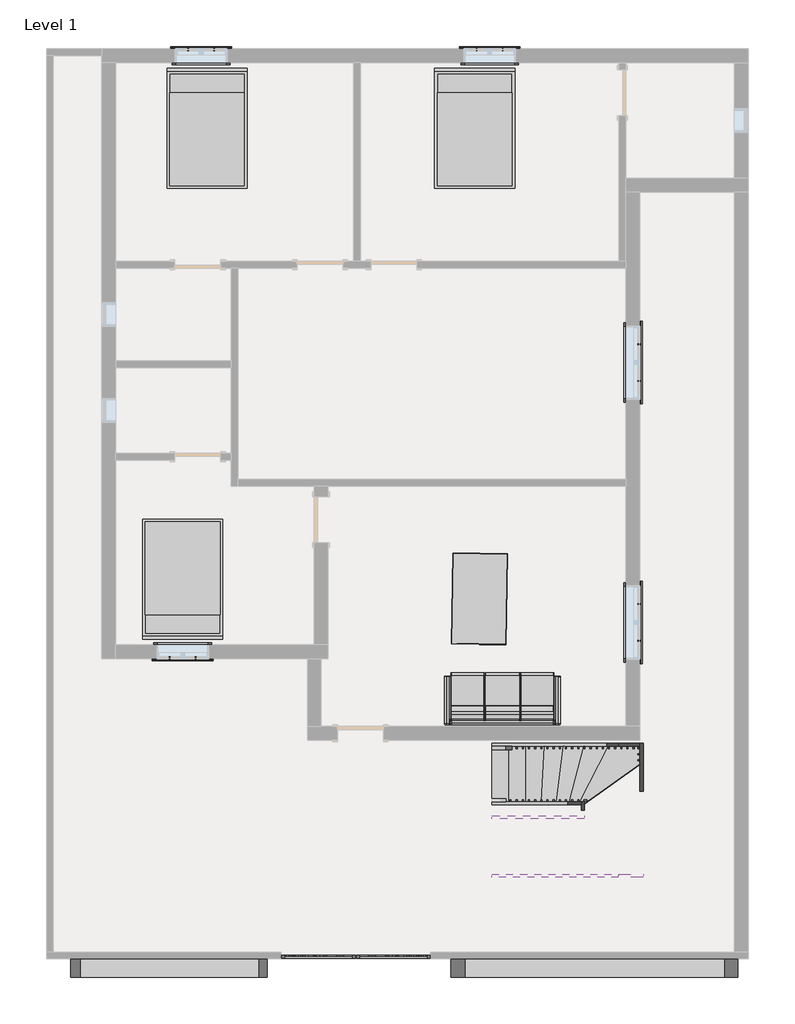
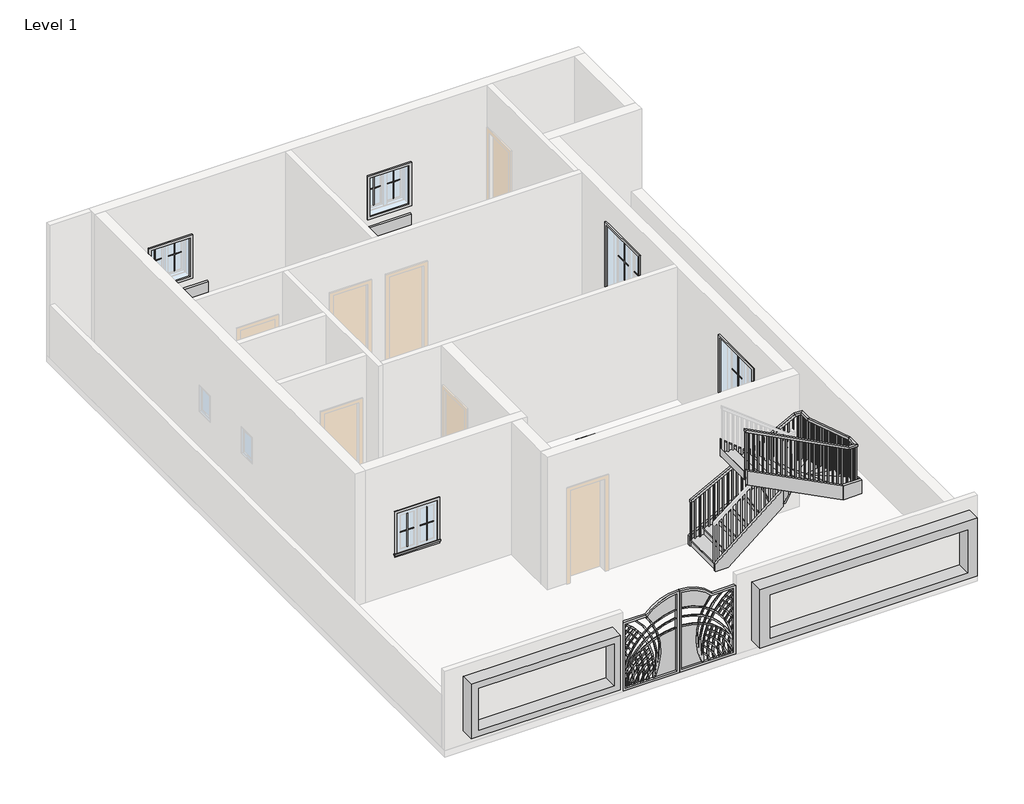
# One storey, part 2 of 2: 23 proxies, 8 members, 5 furniture elements, 1 railing, 1 stair flight.
"""IFC4 building model written with IfcOpenShell, lengths in millimetres."""

from ifc_helpers import new_model, si_unit, frame, origin, place, context, project, spatial, polyline, outline, extrude, faceted_brep, transform, mapped, element, save
from components import generic_models_6bc30956, generic_models_1_generic_models_1_5f3879a5, generic_models_2_generic_models_2_98d93cec, muntin_pattern_2x2_muntin_pattern_2x2_b3fe6957, muntin_pattern_2x2_muntin_pattern_2x2_3e0ecaf2, muntin_pattern_2x2_muntin_pattern_2x2_6dad3731, muntin_pattern_2x2_muntin_pattern_2x2_a30a3345, trim_window_exterior_flat_with_sill_41619996, trim_window_exterior_flat_with_sill_92b9b949, trim_window_interior_flat_picture_frame_51c85655, trim_window_interior_flat_picture_frame_3bb882cf, furniture_2fc85b74, furniture_29a9adb8, furniture_57072a26, bed_17739_bed_17739_15c61121, dining_table_14755_dining_table_14755_d89cb775, stair_flight_f23435a1

model = new_model("IFC4")

# Units and contexts
model_context = context("Model", 3, world=origin())
ifc_project = project(units=[si_unit("LENGTHUNIT", "METRE", prefix="MILLI")], contexts=[model_context])

# Site, building, storey
site = spatial("IfcSite", under=ifc_project)
building = spatial("IfcBuilding", under=site)
storey = spatial("IfcBuildingStorey", under=building, Name="Level 1", Elevation=0.0)

# Proxies
placement = place(None, origin())
generic_models_shape = generic_models_6bc30956(model_context)
element("IfcBuildingElementProxy", 1, Name="Generic Models", at=placement, inside=storey, context=model_context, shape_type="MappedRepresentation", body=[
    mapped(generic_models_shape, transform((-1944.195824, -6904.0064015, 0.0), x_axis=(1.0, 0.0, 0.0), y_axis=(0.0, 1.0, 0.0), z_axis=(0.0, 0.0, 1.0))),
])
generic_models_1_generic_models_1_shape = generic_models_1_generic_models_1_5f3879a5(model_context)
element("IfcBuildingElementProxy", 2, Name="Generic Models 1 : Generic Models 1", ObjectType="Generic Models 1 : Generic Models 1", at=placement, inside=storey, context=model_context, shape_type="MappedRepresentation", body=[
    mapped(generic_models_1_generic_models_1_shape, transform((0.0, 0.0, 0.0), x_axis=(1.0, 0.0, 0.0), y_axis=(0.0, 1.0, 0.0), z_axis=(0.0, 0.0, 1.0))),
])
generic_models_2_generic_models_2_shape = generic_models_2_generic_models_2_98d93cec(model_context)
element("IfcBuildingElementProxy", 3, Name="Generic Models 2 : Generic Models 2", ObjectType="Generic Models 2 : Generic Models 2", at=placement, inside=storey, context=model_context, shape_type="MappedRepresentation", body=[
    mapped(generic_models_2_generic_models_2_shape, transform((0.0, 0.0, 0.0), x_axis=(1.0, 0.0, 0.0), y_axis=(0.0, 1.0, 0.0), z_axis=(0.0, 0.0, 1.0))),
])
muntin_pattern_2x2_muntin_pattern_2x2_shape = muntin_pattern_2x2_muntin_pattern_2x2_b3fe6957(model_context)
element("IfcBuildingElementProxy", 4, Name="Muntin Pattern_2x2 : Muntin Pattern_2x2", ObjectType="Muntin Pattern_2x2 : Muntin Pattern_2x2", at=placement, inside=storey, context=model_context, shape_type="MappedRepresentation", body=[
    mapped(muntin_pattern_2x2_muntin_pattern_2x2_shape, transform((-4708.0540084, 8034.3685985, 984.25), x_axis=(1.0, 0.0, 0.0), y_axis=(0.0, 1.0, 0.0), z_axis=(0.0, 0.0, 1.0))),
])
element("IfcBuildingElementProxy", 5, Name="Muntin Pattern_2x2 : Muntin Pattern_2x2", ObjectType="Muntin Pattern_2x2 : Muntin Pattern_2x2", at=placement, inside=storey, context=model_context, shape_type="MappedRepresentation", body=[
    mapped(muntin_pattern_2x2_muntin_pattern_2x2_shape, transform((54.4459916, 8034.3685985, 984.25), x_axis=(1.0, 0.0, 0.0), y_axis=(0.0, 1.0, 0.0), z_axis=(0.0, 0.0, 1.0))),
])
element("IfcBuildingElementProxy", 6, Name="Muntin Pattern_2x2 : Muntin Pattern_2x2", ObjectType="Muntin Pattern_2x2 : Muntin Pattern_2x2", at=placement, inside=storey, context=model_context, shape_type="MappedRepresentation", body=[
    mapped(muntin_pattern_2x2_muntin_pattern_2x2_shape, transform((-4584.2290084, -2004.9814015, 984.25), x_axis=(-1.0, 0.0, 0.0), y_axis=(0.0, -1.0, 0.0), z_axis=(0.0, 0.0, 1.0))),
])
muntin_pattern_2x2_muntin_pattern_2x2_2_shape = muntin_pattern_2x2_muntin_pattern_2x2_3e0ecaf2(model_context)
element("IfcBuildingElementProxy", 7, Name="Muntin Pattern_2x2 : Muntin Pattern_2x2", ObjectType="Muntin Pattern_2x2 : Muntin Pattern_2x2", at=placement, inside=storey, context=model_context, shape_type="MappedRepresentation", body=[
    mapped(muntin_pattern_2x2_muntin_pattern_2x2_2_shape, transform((-4279.4290084, 8034.3685985, 984.25), x_axis=(-1.0, 0.0, 0.0), y_axis=(0.0, -1.0, 0.0), z_axis=(0.0, 0.0, 1.0))),
])
element("IfcBuildingElementProxy", 8, Name="Muntin Pattern_2x2 : Muntin Pattern_2x2", ObjectType="Muntin Pattern_2x2 : Muntin Pattern_2x2", at=placement, inside=storey, context=model_context, shape_type="MappedRepresentation", body=[
    mapped(muntin_pattern_2x2_muntin_pattern_2x2_2_shape, transform((483.0709916, 8034.3685985, 984.25), x_axis=(-1.0, 0.0, 0.0), y_axis=(0.0, -1.0, 0.0), z_axis=(0.0, 0.0, 1.0))),
])
element("IfcBuildingElementProxy", 9, Name="Muntin Pattern_2x2 : Muntin Pattern_2x2", ObjectType="Muntin Pattern_2x2 : Muntin Pattern_2x2", at=placement, inside=storey, context=model_context, shape_type="MappedRepresentation", body=[
    mapped(muntin_pattern_2x2_muntin_pattern_2x2_2_shape, transform((-5012.8540084, -2004.9814015, 984.25), x_axis=(1.0, 0.0, 0.0), y_axis=(0.0, 1.0, 0.0), z_axis=(0.0, 0.0, 1.0))),
])
muntin_pattern_2x2_muntin_pattern_2x2_3_shape = muntin_pattern_2x2_muntin_pattern_2x2_6dad3731(model_context)
element("IfcBuildingElementProxy", 10, Name="Muntin Pattern_2x2 : Muntin Pattern_2x2", ObjectType="Muntin Pattern_2x2 : Muntin Pattern_2x2", at=placement, inside=storey, context=model_context, shape_type="MappedRepresentation", body=[
    mapped(muntin_pattern_2x2_muntin_pattern_2x2_3_shape, transform((2735.7334916, -1114.3939015, 984.25), x_axis=(0.0, -1.0, 0.0), y_axis=(1.0, 0.0, 0.0), z_axis=(0.0, 0.0, 1.0))),
])
element("IfcBuildingElementProxy", 11, Name="Muntin Pattern_2x2 : Muntin Pattern_2x2", ObjectType="Muntin Pattern_2x2 : Muntin Pattern_2x2", at=placement, inside=storey, context=model_context, shape_type="MappedRepresentation", body=[
    mapped(muntin_pattern_2x2_muntin_pattern_2x2_3_shape, transform((2735.7334916, 3171.8560985, 984.25), x_axis=(0.0, -1.0, 0.0), y_axis=(1.0, 0.0, 0.0), z_axis=(0.0, 0.0, 1.0))),
])
muntin_pattern_2x2_muntin_pattern_2x2_4_shape = muntin_pattern_2x2_muntin_pattern_2x2_a30a3345(model_context)
element("IfcBuildingElementProxy", 12, Name="Muntin Pattern_2x2 : Muntin Pattern_2x2", ObjectType="Muntin Pattern_2x2 : Muntin Pattern_2x2", at=placement, inside=storey, context=model_context, shape_type="MappedRepresentation", body=[
    mapped(muntin_pattern_2x2_muntin_pattern_2x2_4_shape, transform((2735.7334916, -1720.8189015, 984.25), x_axis=(0.0, 1.0, 0.0), y_axis=(-1.0, 0.0, 0.0), z_axis=(0.0, 0.0, 1.0))),
])
element("IfcBuildingElementProxy", 13, Name="Muntin Pattern_2x2 : Muntin Pattern_2x2", ObjectType="Muntin Pattern_2x2 : Muntin Pattern_2x2", at=placement, inside=storey, context=model_context, shape_type="MappedRepresentation", body=[
    mapped(muntin_pattern_2x2_muntin_pattern_2x2_4_shape, transform((2735.7334916, 2565.4310985, 984.25), x_axis=(0.0, 1.0, 0.0), y_axis=(-1.0, 0.0, 0.0), z_axis=(0.0, 0.0, 1.0))),
])
trim_window_exterior_flat_with_sill_shape = trim_window_exterior_flat_with_sill_41619996(model_context)
element("IfcBuildingElementProxy", 14, Name="Trim-Window-Exterior-Flat : with Sill", ObjectType="Trim-Window-Exterior-Flat : with Sill", at=placement, inside=storey, context=model_context, shape_type="MappedRepresentation", body=[
    mapped(trim_window_exterior_flat_with_sill_shape, transform((-4493.7415084, 8043.8935985, 1828.8), x_axis=(-1.0, 0.0, 0.0), y_axis=(0.0, 0.0, 1.0), z_axis=(0.0, 1.0, 0.0))),
])
element("IfcBuildingElementProxy", 15, Name="Trim-Window-Exterior-Flat : with Sill", ObjectType="Trim-Window-Exterior-Flat : with Sill", at=placement, inside=storey, context=model_context, shape_type="MappedRepresentation", body=[
    mapped(trim_window_exterior_flat_with_sill_shape, transform((268.7584916, 8043.8935985, 1828.8), x_axis=(-1.0, 0.0, 0.0), y_axis=(0.0, 0.0, 1.0), z_axis=(0.0, 1.0, 0.0))),
])
element("IfcBuildingElementProxy", 16, Name="Trim-Window-Exterior-Flat : with Sill", ObjectType="Trim-Window-Exterior-Flat : with Sill", at=placement, inside=storey, context=model_context, shape_type="MappedRepresentation", body=[
    mapped(trim_window_exterior_flat_with_sill_shape, transform((-4798.5415084, -2014.5064015, 1828.8), x_axis=(1.0, 0.0, 0.0), y_axis=(0.0, 0.0, 1.0), z_axis=(0.0, -1.0, 0.0))),
])
trim_window_exterior_flat_with_sill_2_shape = trim_window_exterior_flat_with_sill_92b9b949(model_context)
element("IfcBuildingElementProxy", 17, Name="Trim-Window-Exterior-Flat : with Sill", ObjectType="Trim-Window-Exterior-Flat : with Sill", at=placement, inside=storey, context=model_context, shape_type="MappedRepresentation", body=[
    mapped(trim_window_exterior_flat_with_sill_2_shape, transform((2745.2584916, -1417.6064015, 2438.4), x_axis=(0.0, 1.0, 0.0), y_axis=(0.0, 0.0, 1.0), z_axis=(1.0, 0.0, 0.0))),
])
element("IfcBuildingElementProxy", 18, Name="Trim-Window-Exterior-Flat : with Sill", ObjectType="Trim-Window-Exterior-Flat : with Sill", at=placement, inside=storey, context=model_context, shape_type="MappedRepresentation", body=[
    mapped(trim_window_exterior_flat_with_sill_2_shape, transform((2745.2584916, 2868.6435985, 2438.4), x_axis=(0.0, 1.0, 0.0), y_axis=(0.0, 0.0, 1.0), z_axis=(1.0, 0.0, 0.0))),
])
trim_window_interior_flat_picture_frame_shape = trim_window_interior_flat_picture_frame_51c85655(model_context)
element("IfcBuildingElementProxy", 19, Name="Trim-Window-Interior-Flat : Picture Frame", ObjectType="Trim-Window-Interior-Flat : Picture Frame", at=placement, inside=storey, context=model_context, shape_type="MappedRepresentation", body=[
    mapped(trim_window_interior_flat_picture_frame_shape, transform((-4493.7415084, 7815.2935985, 1828.8), x_axis=(1.0, 0.0, 0.0), y_axis=(0.0, 0.0, 1.0), z_axis=(0.0, -1.0, 0.0))),
])
element("IfcBuildingElementProxy", 20, Name="Trim-Window-Interior-Flat : Picture Frame", ObjectType="Trim-Window-Interior-Flat : Picture Frame", at=placement, inside=storey, context=model_context, shape_type="MappedRepresentation", body=[
    mapped(trim_window_interior_flat_picture_frame_shape, transform((268.7584916, 7815.2935985, 1828.8), x_axis=(1.0, 0.0, 0.0), y_axis=(0.0, 0.0, 1.0), z_axis=(0.0, -1.0, 0.0))),
])
element("IfcBuildingElementProxy", 21, Name="Trim-Window-Interior-Flat : Picture Frame", ObjectType="Trim-Window-Interior-Flat : Picture Frame", at=placement, inside=storey, context=model_context, shape_type="MappedRepresentation", body=[
    mapped(trim_window_interior_flat_picture_frame_shape, transform((-4798.5415084, -1785.9064015, 1828.8), x_axis=(-1.0, 0.0, 0.0), y_axis=(0.0, 0.0, 1.0), z_axis=(0.0, 1.0, 0.0))),
])
trim_window_interior_flat_picture_frame_2_shape = trim_window_interior_flat_picture_frame_3bb882cf(model_context)
element("IfcBuildingElementProxy", 22, Name="Trim-Window-Interior-Flat : Picture Frame", ObjectType="Trim-Window-Interior-Flat : Picture Frame", at=placement, inside=storey, context=model_context, shape_type="MappedRepresentation", body=[
    mapped(trim_window_interior_flat_picture_frame_2_shape, transform((2516.6584916, -1417.6064015, 2438.4), x_axis=(0.0, -1.0, 0.0), y_axis=(0.0, 0.0, 1.0), z_axis=(-1.0, 0.0, 0.0))),
])
element("IfcBuildingElementProxy", 23, Name="Trim-Window-Interior-Flat : Picture Frame", ObjectType="Trim-Window-Interior-Flat : Picture Frame", at=placement, inside=storey, context=model_context, shape_type="MappedRepresentation", body=[
    mapped(trim_window_interior_flat_picture_frame_2_shape, transform((2516.6584916, 2868.6435985, 2438.4), x_axis=(0.0, -1.0, 0.0), y_axis=(0.0, 0.0, 1.0), z_axis=(-1.0, 0.0, 0.0))),
])

# Furniture
furniture_shape = furniture_2fc85b74(model_context)
furniture_2_shape = furniture_29a9adb8(model_context)
furniture_3_shape = furniture_57072a26(model_context)
element("IfcFurniture", 24, at=placement, inside=storey, context=model_context, shape_type="MappedRepresentation", body=[
    mapped(furniture_shape, transform((477.9947981, -2301.7922014, 0.0), x_axis=(-1.0, 0.0, 0.0), y_axis=(0.0, -1.0, 0.0), z_axis=(0.0, 0.0, 1.0))),
    mapped(furniture_2_shape, transform((477.9947981, -2301.7922014, 0.0), x_axis=(-1.0, 0.0, 0.0), y_axis=(0.0, -1.0, 0.0), z_axis=(0.0, 0.0, 1.0))),
    mapped(furniture_3_shape, transform((477.9947981, -2301.7922014, 0.0), x_axis=(-1.0, 0.0, 0.0), y_axis=(0.0, -1.0, 0.0), z_axis=(0.0, 0.0, 1.0))),
])
bed_17739_bed_17739_shape = bed_17739_bed_17739_15c61121(model_context)
element("IfcFurniture", 25, ObjectType="Bed_17739 : Bed_17739", at=placement, inside=storey, context=model_context, shape_type="MappedRepresentation", body=[
    mapped(bed_17739_bed_17739_shape, transform((-4398.4915084, 6710.3935985, 0.0), x_axis=(1.0, 0.0, 0.0), y_axis=(0.0, 1.0, 0.0), z_axis=(0.0, 0.0, 1.0))),
])
element("IfcFurniture", 26, ObjectType="Bed_17739 : Bed_17739", at=placement, inside=storey, context=model_context, shape_type="MappedRepresentation", body=[
    mapped(bed_17739_bed_17739_shape, transform((21.1084916, 6710.3935985, 0.0), x_axis=(1.0, 0.0, 0.0), y_axis=(0.0, 1.0, 0.0), z_axis=(0.0, 0.0, 1.0))),
])
element("IfcFurniture", 27, ObjectType="Bed_17739 : Bed_17739", at=placement, inside=storey, context=model_context, shape_type="MappedRepresentation", body=[
    mapped(bed_17739_bed_17739_shape, transform((-4798.5415084, -681.0064015, 0.0), x_axis=(-1.0, 0.0, 0.0), y_axis=(0.0, -1.0, 0.0), z_axis=(0.0, 0.0, 1.0))),
])
dining_table_14755_dining_table_14755_shape = dining_table_14755_dining_table_14755_d89cb775(model_context)
element("IfcFurniture", 28, ObjectType="Dining_table_14755 : Dining_table_14755", at=placement, inside=storey, context=model_context, shape_type="MappedRepresentation", body=[
    mapped(dining_table_14755_dining_table_14755_shape, transform((535.647979, -1785.9064015, 0.0), x_axis=(0.016088397262737867, 0.9998705733611308, 0.0), y_axis=(-0.9998705733611308, 0.016088397262737867, 0.0), z_axis=(0.0, 0.0, 1.0))),
])

# Members
element("IfcMember", 29, ObjectType="Stringer - 2\" Width", at=placement, inside=storey, context=model_context, shape_type="SweptSolid", body=[
    extrude(outline(polyline([(229.639954, 306.9570026), (0.0, 306.9570026), (0.0, 526.7193201), (962.500629, 2394.3741942), (1305.3956453, 2394.3741942), (229.639954, 306.9570026)])), frame((0.0, -3462.3064015, 0.0), z_axis=(0.0, 1.0, 0.0), x_axis=(0.0, 0.0, 1.0)), (0.0, 0.0, 1.0), 50.8),
])
element("IfcMember", 30, ObjectType="Stringer - 2\" Width", at=placement, inside=storey, context=model_context, shape_type="SweptSolid", body=[
    extrude(outline(polyline([(2394.3741942, -3462.3064015), (2394.3741942, -3411.5064015), (2749.0886944, -3411.5064015), (2749.0886944, -3462.3064015), (2394.3741942, -3462.3064015)])), frame((0.0, 0.0, 962.500629), z_axis=(0.0, 0.0, 1.0), x_axis=(1.0, 0.0, 0.0)), (0.0, 0.0, 1.0), 342.8950162),
])
element("IfcMember", 31, ObjectType="Stringer - 2\" Width", at=placement, inside=storey, context=model_context, shape_type="SweptSolid", body=[
    extrude(outline(polyline([(-3411.5064015, 1289.0952212), (-3411.5064015, 1000.5956453), (-3581.0288845, 1000.5956453), (-5570.5064015, 1638.9682298), (-5570.5064015, 1969.9972697), (-5533.5262842, 1969.9972697), (-3411.5064015, 1289.0952212)])), frame((2749.0886944, 0.0, 0.0), z_axis=(1.0, 0.0, 0.0), x_axis=(0.0, 1.0, 0.0)), (0.0, 0.0, 1.0), 50.8),
])
element("IfcMember", 32, ObjectType="Stringer - 2\" Width", at=placement, inside=storey, context=model_context, shape_type="SweptSolid", body=[
    extrude(outline(polyline([(2799.8886944, -5570.5064015), (2799.8886944, -5621.3064015), (2394.3741942, -5621.3064015), (2394.3741942, -5570.5064015), (2799.8886944, -5570.5064015)])), frame((0.0, 0.0, 1649.8904473), z_axis=(0.0, 0.0, 1.0), x_axis=(1.0, 0.0, 0.0)), (0.0, 0.0, 1.0), 320.1068224),
])
element("IfcMember", 33, ObjectType="Stringer - 2\" Width", at=placement, inside=storey, context=model_context, shape_type="SweptSolid", body=[
    extrude(outline(polyline([(1649.8904473, 2394.3741942), (1969.9972697, 2394.3741942), (3045.7529609, 306.9570026), (2725.6461385, 306.9570026), (1649.8904473, 2394.3741942)])), frame((0.0, -5621.3064015, 0.0), z_axis=(0.0, 1.0, 0.0), x_axis=(0.0, 0.0, 1.0)), (0.0, 0.0, 1.0), 50.8),
])
element("IfcMember", 34, ObjectType="Stringer - 2\" Width", at=placement, inside=storey, context=model_context, shape_type="SweptSolid", body=[
    extrude(outline(polyline([(176.1764461, 306.9570026), (0.0, 306.9570026), (0.0, 573.2186471), (987.1410923, 1783.8886944), (1380.418648, 1783.8886944), (176.1764461, 306.9570026)])), frame((0.0, -4427.5064015, 0.0), z_axis=(0.0, 1.0, 0.0), x_axis=(0.0, 0.0, 1.0)), (0.0, 0.0, 1.0), 50.8),
])
element("IfcMember", 35, ObjectType="Stringer - 2\" Width", at=placement, inside=storey, context=model_context, shape_type="SweptSolid", body=[
    extrude(outline(polyline([(-4376.7064015, 1573.2682978), (-4376.7064015, 1028.5617647), (-4410.9486188, 1028.5617647), (-4605.3064015, 1360.465107), (-4605.3064015, 1926.1409689), (-4583.3435189, 1926.1409689), (-4376.7064015, 1573.2682978)])), frame((1783.8886944, 0.0, 0.0), z_axis=(1.0, 0.0, 0.0), x_axis=(0.0, 1.0, 0.0)), (0.0, 0.0, 1.0), 50.8),
])
element("IfcMember", 36, ObjectType="Stringer - 2\" Width", at=placement, inside=storey, context=model_context, shape_type="SweptSolid", body=[
    extrude(outline(polyline([(1532.8634131, 1834.6886944), (1926.1409689, 1834.6886944), (3171.8038432, 306.9570026), (2778.5262875, 306.9570026), (1532.8634131, 1834.6886944)])), frame((0.0, -4656.1064015, 0.0), z_axis=(0.0, 1.0, 0.0), x_axis=(0.0, 0.0, 1.0)), (0.0, 0.0, 1.0), 50.8),
])

# Railing
element("IfcRailing", 37, ObjectType="Handrail - Rectangular", at=placement, inside=storey, context=model_context, shape_type="SolidModel", body=[
    faceted_brep([(306.9570026, -3462.3064015, 1083.7333333), (306.9570026, -3462.3064015, 1026.2742652), (306.9570026, -3513.1064015, 1026.2742652), (306.9570026, -3513.1064015, 1083.7333333), (2564.6820646, -3462.3064015, 2277.0239201), (2577.2811291, -3462.3064015, 2226.2239201), (2577.2811291, -3513.1064015, 2226.2239201), (2564.6820646, -3513.1064015, 2277.0239201), (2749.0886944, -3462.3064015, 2277.0239201), (2749.0886944, -3462.3064015, 2226.2239201), (2698.2886944, -3513.1064015, 2226.2239201), (2698.2886944, -3513.1064015, 2277.0239201), (2749.0886944, -3749.6182836, 2277.0239201), (2749.0886944, -3757.5688598, 2226.2239201), (2698.2886944, -3757.5688598, 2226.2239201), (2698.2886944, -3749.6182836, 2277.0239201), (2749.0886944, -5283.1945194, 2769.1094132), (2749.0886944, -5291.1450955, 2718.3094132), (2698.2886944, -5291.1450955, 2718.3094132), (2698.2886944, -5283.1945194, 2769.1094132), (2749.0886944, -5570.5064015, 2769.1094132), (2749.0886944, -5570.5064015, 2718.3094132), (2698.2886944, -5519.7064015, 2718.3094132), (2698.2886944, -5519.7064015, 2769.1094132), (2564.6820646, -5570.5064015, 2769.1094132), (2552.0830001, -5570.5064015, 2718.3094132), (2552.0830001, -5519.7064015, 2718.3094132), (2564.6820646, -5519.7064015, 2769.1094132), (306.9570026, -5570.5064015, 3962.4), (306.9570026, -5519.7064015, 3962.4), (306.9570026, -5519.7064015, 3904.9409318), (306.9570026, -5570.5064015, 3904.9409318)], [[[0, 1, 2, 3]], [[1, 0, 4, 5]], [[2, 1, 5, 6]], [[3, 2, 6, 7]], [[0, 3, 7, 4]], [[5, 4, 8, 9]], [[6, 5, 9, 10]], [[7, 6, 10, 11]], [[4, 7, 11, 8]], [[9, 8, 12, 13]], [[10, 9, 13, 14]], [[11, 10, 14, 15]], [[8, 11, 15, 12]], [[13, 12, 16, 17]], [[14, 13, 17, 18]], [[15, 14, 18, 19]], [[12, 15, 19, 16]], [[17, 16, 20, 21]], [[18, 17, 21, 22]], [[19, 18, 22, 23]], [[16, 19, 23, 20]], [[21, 20, 24, 25]], [[22, 21, 25, 26]], [[23, 22, 26, 27]], [[20, 23, 27, 24]], [[28, 29, 30, 31]], [[25, 24, 28, 31]], [[26, 25, 31, 30]], [[27, 26, 30, 29]], [[24, 27, 29, 28]]]),
    extrude(outline(polyline([(3867.7284102, 377.3636944), (2878.6666667, 377.3636944), (2878.6666667, 396.4136944), (3857.6597858, 396.4136944), (3867.7284102, 377.3636944)])), frame((0.0, -5554.6314015, 0.0), z_axis=(0.0, 1.0, 0.0), x_axis=(0.0, 0.0, 1.0)), (0.0, 0.0, 1.0), 19.05),
    extrude(outline(polyline([(3814.02908, 478.9636944), (2878.6666667, 478.9636944), (2878.6666667, 498.0136944), (3803.9604556, 498.0136944), (3814.02908, 478.9636944)])), frame((0.0, -5554.6314015, 0.0), z_axis=(0.0, 1.0, 0.0), x_axis=(0.0, 0.0, 1.0)), (0.0, 0.0, 1.0), 19.05),
    extrude(outline(polyline([(3760.3297498, 580.5636944), (2709.3333333, 580.5636944), (2709.3333333, 599.6136944), (3750.2611254, 599.6136944), (3760.3297498, 580.5636944)])), frame((0.0, -5554.6314015, 0.0), z_axis=(0.0, 1.0, 0.0), x_axis=(0.0, 0.0, 1.0)), (0.0, 0.0, 1.0), 19.05),
    extrude(outline(polyline([(3706.6304196, 682.1636944), (2709.3333333, 682.1636944), (2709.3333333, 701.2136944), (3696.5617952, 701.2136944), (3706.6304196, 682.1636944)])), frame((0.0, -5554.6314015, 0.0), z_axis=(0.0, 1.0, 0.0), x_axis=(0.0, 0.0, 1.0)), (0.0, 0.0, 1.0), 19.05),
    extrude(outline(polyline([(3652.9310894, 783.7636944), (2709.3333333, 783.7636944), (2709.3333333, 802.8136944), (3642.862465, 802.8136944), (3652.9310894, 783.7636944)])), frame((0.0, -5554.6314015, 0.0), z_axis=(0.0, 1.0, 0.0), x_axis=(0.0, 0.0, 1.0)), (0.0, 0.0, 1.0), 19.05),
    extrude(outline(polyline([(3599.2317592, 885.3636944), (2540.0, 885.3636944), (2540.0, 904.4136944), (3589.1631348, 904.4136944), (3599.2317592, 885.3636944)])), frame((0.0, -5554.6314015, 0.0), z_axis=(0.0, 1.0, 0.0), x_axis=(0.0, 0.0, 1.0)), (0.0, 0.0, 1.0), 19.05),
    extrude(outline(polyline([(3545.532429, 986.9636944), (2540.0, 986.9636944), (2540.0, 1006.0136944), (3535.4638046, 1006.0136944), (3545.532429, 986.9636944)])), frame((0.0, -5554.6314015, 0.0), z_axis=(0.0, 1.0, 0.0), x_axis=(0.0, 0.0, 1.0)), (0.0, 0.0, 1.0), 19.05),
    extrude(outline(polyline([(3491.8330988, 1088.5636944), (2540.0, 1088.5636944), (2540.0, 1107.6136944), (3481.7644744, 1107.6136944), (3491.8330988, 1088.5636944)])), frame((0.0, -5554.6314015, 0.0), z_axis=(0.0, 1.0, 0.0), x_axis=(0.0, 0.0, 1.0)), (0.0, 0.0, 1.0), 19.05),
    extrude(outline(polyline([(3438.1337686, 1190.1636944), (2370.6666667, 1190.1636944), (2370.6666667, 1209.2136944), (3428.0651442, 1209.2136944), (3438.1337686, 1190.1636944)])), frame((0.0, -5554.6314015, 0.0), z_axis=(0.0, 1.0, 0.0), x_axis=(0.0, 0.0, 1.0)), (0.0, 0.0, 1.0), 19.05),
    extrude(outline(polyline([(3384.4344384, 1291.7636944), (2370.6666667, 1291.7636944), (2370.6666667, 1310.8136944), (3374.365814, 1310.8136944), (3384.4344384, 1291.7636944)])), frame((0.0, -5554.6314015, 0.0), z_axis=(0.0, 1.0, 0.0), x_axis=(0.0, 0.0, 1.0)), (0.0, 0.0, 1.0), 19.05),
    extrude(outline(polyline([(3330.7351082, 1393.3636944), (2370.6666667, 1393.3636944), (2370.6666667, 1412.4136944), (3320.6664838, 1412.4136944), (3330.7351082, 1393.3636944)])), frame((0.0, -5554.6314015, 0.0), z_axis=(0.0, 1.0, 0.0), x_axis=(0.0, 0.0, 1.0)), (0.0, 0.0, 1.0), 19.05),
    extrude(outline(polyline([(3277.035778, 1494.9636944), (2201.3333333, 1494.9636944), (2201.3333333, 1514.0136944), (3266.9671536, 1514.0136944), (3277.035778, 1494.9636944)])), frame((0.0, -5554.6314015, 0.0), z_axis=(0.0, 1.0, 0.0), x_axis=(0.0, 0.0, 1.0)), (0.0, 0.0, 1.0), 19.05),
    extrude(outline(polyline([(3223.3364478, 1596.5636944), (2201.3333333, 1596.5636944), (2201.3333333, 1615.6136944), (3213.2678234, 1615.6136944), (3223.3364478, 1596.5636944)])), frame((0.0, -5554.6314015, 0.0), z_axis=(0.0, 1.0, 0.0), x_axis=(0.0, 0.0, 1.0)), (0.0, 0.0, 1.0), 19.05),
    extrude(outline(polyline([(3169.6371176, 1698.1636944), (2201.3333333, 1698.1636944), (2201.3333333, 1717.2136944), (3159.5684932, 1717.2136944), (3169.6371176, 1698.1636944)])), frame((0.0, -5554.6314015, 0.0), z_axis=(0.0, 1.0, 0.0), x_axis=(0.0, 0.0, 1.0)), (0.0, 0.0, 1.0), 19.05),
    extrude(outline(polyline([(3115.9377874, 1799.7636944), (2201.3333333, 1799.7636944), (2201.3333333, 1818.8136944), (3105.869163, 1818.8136944), (3115.9377874, 1799.7636944)])), frame((0.0, -5554.6314015, 0.0), z_axis=(0.0, 1.0, 0.0), x_axis=(0.0, 0.0, 1.0)), (0.0, 0.0, 1.0), 19.05),
    extrude(outline(polyline([(3062.2384572, 1901.3636944), (2032.0, 1901.3636944), (2032.0, 1920.4136944), (3052.1698328, 1920.4136944), (3062.2384572, 1901.3636944)])), frame((0.0, -5554.6314015, 0.0), z_axis=(0.0, 1.0, 0.0), x_axis=(0.0, 0.0, 1.0)), (0.0, 0.0, 1.0), 19.05),
    extrude(outline(polyline([(3008.539127, 2002.9636944), (2032.0, 2002.9636944), (2032.0, 2022.0136944), (2998.4705026, 2022.0136944), (3008.539127, 2002.9636944)])), frame((0.0, -5554.6314015, 0.0), z_axis=(0.0, 1.0, 0.0), x_axis=(0.0, 0.0, 1.0)), (0.0, 0.0, 1.0), 19.05),
    extrude(outline(polyline([(2954.8397968, 2104.5636944), (2032.0, 2104.5636944), (2032.0, 2123.6136944), (2944.7711724, 2123.6136944), (2954.8397968, 2104.5636944)])), frame((0.0, -5554.6314015, 0.0), z_axis=(0.0, 1.0, 0.0), x_axis=(0.0, 0.0, 1.0)), (0.0, 0.0, 1.0), 19.05),
    extrude(outline(polyline([(2901.1404666, 2206.1636944), (2032.0, 2206.1636944), (2032.0, 2225.2136944), (2891.0718422, 2225.2136944), (2901.1404666, 2206.1636944)])), frame((0.0, -5554.6314015, 0.0), z_axis=(0.0, 1.0, 0.0), x_axis=(0.0, 0.0, 1.0)), (0.0, 0.0, 1.0), 19.05),
    extrude(outline(polyline([(2847.4411364, 2307.7636944), (1862.6666667, 2307.7636944), (1862.6666667, 2326.8136944), (2837.372512, 2326.8136944), (2847.4411364, 2307.7636944)])), frame((0.0, -5554.6314015, 0.0), z_axis=(0.0, 1.0, 0.0), x_axis=(0.0, 0.0, 1.0)), (0.0, 0.0, 1.0), 19.05),
    extrude(outline(polyline([(2793.7418062, 2409.3636944), (1862.6666667, 2409.3636944), (1862.6666667, 2428.4136944), (2783.6731818, 2428.4136944), (2793.7418062, 2409.3636944)])), frame((0.0, -5554.6314015, 0.0), z_axis=(0.0, 1.0, 0.0), x_axis=(0.0, 0.0, 1.0)), (0.0, 0.0, 1.0), 19.05),
    extrude(outline(polyline([(2740.042476, 2510.9636944), (1862.6666667, 2510.9636944), (1862.6666667, 2530.0136944), (2729.9738516, 2530.0136944), (2740.042476, 2510.9636944)])), frame((0.0, -5554.6314015, 0.0), z_axis=(0.0, 1.0, 0.0), x_axis=(0.0, 0.0, 1.0)), (0.0, 0.0, 1.0), 19.05),
    extrude(outline(polyline([(2631.6136944, -5554.6314015), (2612.5636944, -5554.6314015), (2612.5636944, -5535.5814015), (2631.6136944, -5535.5814015), (2631.6136944, -5554.6314015)])), frame((0.0, 0.0, 1862.6666667), z_axis=(0.0, 0.0, 1.0), x_axis=(1.0, 0.0, 0.0)), (0.0, 0.0, 1.0), 855.6427466),
    extrude(outline(polyline([(2733.2136944, -5510.1814015), (2733.2136944, -5529.2314015), (2714.1636944, -5529.2314015), (2714.1636944, -5510.1814015), (2733.2136944, -5510.1814015)])), frame((0.0, 0.0, 1862.6666667), z_axis=(0.0, 0.0, 1.0), x_axis=(1.0, 0.0, 0.0)), (0.0, 0.0, 1.0), 855.6427466),
    extrude(outline(polyline([(2733.2136944, -5408.5814015), (2733.2136944, -5427.6314015), (2714.1636944, -5427.6314015), (2714.1636944, -5408.5814015), (2733.2136944, -5408.5814015)])), frame((0.0, 0.0, 1862.6666667), z_axis=(0.0, 0.0, 1.0), x_axis=(1.0, 0.0, 0.0)), (0.0, 0.0, 1.0), 855.6427466),
    extrude(outline(polyline([(2733.2136944, -5306.9814015), (2733.2136944, -5326.0314015), (2714.1636944, -5326.0314015), (2714.1636944, -5306.9814015), (2733.2136944, -5306.9814015)])), frame((0.0, 0.0, 1862.6666667), z_axis=(0.0, 0.0, 1.0), x_axis=(1.0, 0.0, 0.0)), (0.0, 0.0, 1.0), 855.6427466),
    extrude(outline(polyline([(-5205.3814015, 2690.7900316), (-5205.3814015, 1693.3333333), (-5224.4314015, 1693.3333333), (-5224.4314015, 2696.9026907), (-5205.3814015, 2690.7900316)])), frame((2714.1636944, 0.0, 0.0), z_axis=(1.0, 0.0, 0.0), x_axis=(0.0, 1.0, 0.0)), (0.0, 0.0, 1.0), 19.05),
    extrude(outline(polyline([(-5103.7814015, 2658.1891834), (-5103.7814015, 1693.3333333), (-5122.8314015, 1693.3333333), (-5122.8314015, 2664.3018425), (-5103.7814015, 2658.1891834)])), frame((2714.1636944, 0.0, 0.0), z_axis=(1.0, 0.0, 0.0), x_axis=(0.0, 1.0, 0.0)), (0.0, 0.0, 1.0), 19.05),
    extrude(outline(polyline([(-5002.1814015, 2625.5883352), (-5002.1814015, 1693.3333333), (-5021.2314015, 1693.3333333), (-5021.2314015, 2631.7009942), (-5002.1814015, 2625.5883352)])), frame((2714.1636944, 0.0, 0.0), z_axis=(1.0, 0.0, 0.0), x_axis=(0.0, 1.0, 0.0)), (0.0, 0.0, 1.0), 19.05),
    extrude(outline(polyline([(-4900.5814015, 2592.987487), (-4900.5814015, 1693.3333333), (-4919.6314015, 1693.3333333), (-4919.6314015, 2599.100146), (-4900.5814015, 2592.987487)])), frame((2714.1636944, 0.0, 0.0), z_axis=(1.0, 0.0, 0.0), x_axis=(0.0, 1.0, 0.0)), (0.0, 0.0, 1.0), 19.05),
    extrude(outline(polyline([(-4798.9814015, 2560.3866387), (-4798.9814015, 1693.3333333), (-4818.0314015, 1693.3333333), (-4818.0314015, 2566.4992978), (-4798.9814015, 2560.3866387)])), frame((2714.1636944, 0.0, 0.0), z_axis=(1.0, 0.0, 0.0), x_axis=(0.0, 1.0, 0.0)), (0.0, 0.0, 1.0), 19.05),
    extrude(outline(polyline([(-4697.3814015, 2527.7857905), (-4697.3814015, 1524.0), (-4716.4314015, 1524.0), (-4716.4314015, 2533.8984495), (-4697.3814015, 2527.7857905)])), frame((2714.1636944, 0.0, 0.0), z_axis=(1.0, 0.0, 0.0), x_axis=(0.0, 1.0, 0.0)), (0.0, 0.0, 1.0), 19.05),
    extrude(outline(polyline([(-4595.7814015, 2495.1849423), (-4595.7814015, 1524.0), (-4614.8314015, 1524.0), (-4614.8314015, 2501.2976013), (-4595.7814015, 2495.1849423)])), frame((2714.1636944, 0.0, 0.0), z_axis=(1.0, 0.0, 0.0), x_axis=(0.0, 1.0, 0.0)), (0.0, 0.0, 1.0), 19.05),
    extrude(outline(polyline([(-4494.1814015, 2462.5840941), (-4494.1814015, 1524.0), (-4513.2314015, 1524.0), (-4513.2314015, 2468.6967531), (-4494.1814015, 2462.5840941)])), frame((2714.1636944, 0.0, 0.0), z_axis=(1.0, 0.0, 0.0), x_axis=(0.0, 1.0, 0.0)), (0.0, 0.0, 1.0), 19.05),
    extrude(outline(polyline([(-4392.5814015, 2429.9832458), (-4392.5814015, 1524.0), (-4411.6314015, 1524.0), (-4411.6314015, 2436.0959049), (-4392.5814015, 2429.9832458)])), frame((2714.1636944, 0.0, 0.0), z_axis=(1.0, 0.0, 0.0), x_axis=(0.0, 1.0, 0.0)), (0.0, 0.0, 1.0), 19.05),
    extrude(outline(polyline([(-4290.9814015, 2397.3823976), (-4290.9814015, 1524.0), (-4310.0314015, 1524.0), (-4310.0314015, 2403.4950566), (-4290.9814015, 2397.3823976)])), frame((2714.1636944, 0.0, 0.0), z_axis=(1.0, 0.0, 0.0), x_axis=(0.0, 1.0, 0.0)), (0.0, 0.0, 1.0), 19.05),
    extrude(outline(polyline([(-4189.3814015, 2364.7815494), (-4189.3814015, 1354.6666667), (-4208.4314015, 1354.6666667), (-4208.4314015, 2370.8942084), (-4189.3814015, 2364.7815494)])), frame((2714.1636944, 0.0, 0.0), z_axis=(1.0, 0.0, 0.0), x_axis=(0.0, 1.0, 0.0)), (0.0, 0.0, 1.0), 19.05),
    extrude(outline(polyline([(-4087.7814015, 2332.1807011), (-4087.7814015, 1354.6666667), (-4106.8314015, 1354.6666667), (-4106.8314015, 2338.2933602), (-4087.7814015, 2332.1807011)])), frame((2714.1636944, 0.0, 0.0), z_axis=(1.0, 0.0, 0.0), x_axis=(0.0, 1.0, 0.0)), (0.0, 0.0, 1.0), 19.05),
    extrude(outline(polyline([(-3986.1814015, 2299.5798529), (-3986.1814015, 1354.6666667), (-4005.2314015, 1354.6666667), (-4005.2314015, 2305.692512), (-3986.1814015, 2299.5798529)])), frame((2714.1636944, 0.0, 0.0), z_axis=(1.0, 0.0, 0.0), x_axis=(0.0, 1.0, 0.0)), (0.0, 0.0, 1.0), 19.05),
    extrude(outline(polyline([(-3884.5814015, 2266.9790047), (-3884.5814015, 1354.6666667), (-3903.6314015, 1354.6666667), (-3903.6314015, 2273.0916637), (-3884.5814015, 2266.9790047)])), frame((2714.1636944, 0.0, 0.0), z_axis=(1.0, 0.0, 0.0), x_axis=(0.0, 1.0, 0.0)), (0.0, 0.0, 1.0), 19.05),
    extrude(outline(polyline([(-3782.9814015, 2234.3781565), (-3782.9814015, 1354.6666667), (-3802.0314015, 1354.6666667), (-3802.0314015, 2240.4908155), (-3782.9814015, 2234.3781565)])), frame((2714.1636944, 0.0, 0.0), z_axis=(1.0, 0.0, 0.0), x_axis=(0.0, 1.0, 0.0)), (0.0, 0.0, 1.0), 19.05),
    extrude(outline(polyline([(2733.2136944, -3681.3814015), (2733.2136944, -3700.4314015), (2714.1636944, -3700.4314015), (2714.1636944, -3681.3814015), (2733.2136944, -3681.3814015)])), frame((0.0, 0.0, 1185.3333333), z_axis=(0.0, 0.0, 1.0), x_axis=(1.0, 0.0, 0.0)), (0.0, 0.0, 1.0), 1040.8905868),
    extrude(outline(polyline([(2733.2136944, -3579.7814015), (2733.2136944, -3598.8314015), (2714.1636944, -3598.8314015), (2714.1636944, -3579.7814015), (2733.2136944, -3579.7814015)])), frame((0.0, 0.0, 1185.3333333), z_axis=(0.0, 0.0, 1.0), x_axis=(1.0, 0.0, 0.0)), (0.0, 0.0, 1.0), 1040.8905868),
    extrude(outline(polyline([(2634.2320026, -3478.1814015), (2653.2820026, -3478.1814015), (2653.2820026, -3497.2314015), (2634.2320026, -3497.2314015), (2634.2320026, -3478.1814015)])), frame((0.0, 0.0, 1185.3333333), z_axis=(0.0, 0.0, 1.0), x_axis=(1.0, 0.0, 0.0)), (0.0, 0.0, 1.0), 1040.8905868),
    extrude(outline(polyline([(2202.6252174, 2532.6320026), (1185.3333333, 2532.6320026), (1185.3333333, 2551.6820026), (2212.6938418, 2551.6820026), (2202.6252174, 2532.6320026)])), frame((0.0, -3497.2314015, 0.0), z_axis=(0.0, 1.0, 0.0), x_axis=(0.0, 0.0, 1.0)), (0.0, 0.0, 1.0), 19.05),
    extrude(outline(polyline([(2148.9258872, 2431.0320026), (1185.3333333, 2431.0320026), (1185.3333333, 2450.0820026), (2158.9945116, 2450.0820026), (2148.9258872, 2431.0320026)])), frame((0.0, -3497.2314015, 0.0), z_axis=(0.0, 1.0, 0.0), x_axis=(0.0, 0.0, 1.0)), (0.0, 0.0, 1.0), 19.05),
    extrude(outline(polyline([(2095.226557, 2329.4320026), (1185.3333333, 2329.4320026), (1185.3333333, 2348.4820026), (2105.2951814, 2348.4820026), (2095.226557, 2329.4320026)])), frame((0.0, -3497.2314015, 0.0), z_axis=(0.0, 1.0, 0.0), x_axis=(0.0, 0.0, 1.0)), (0.0, 0.0, 1.0), 19.05),
    extrude(outline(polyline([(2041.5272268, 2227.8320026), (1185.3333333, 2227.8320026), (1185.3333333, 2246.8820026), (2051.5958512, 2246.8820026), (2041.5272268, 2227.8320026)])), frame((0.0, -3497.2314015, 0.0), z_axis=(0.0, 1.0, 0.0), x_axis=(0.0, 0.0, 1.0)), (0.0, 0.0, 1.0), 19.05),
    extrude(outline(polyline([(1987.8278966, 2126.2320026), (1016.0, 2126.2320026), (1016.0, 2145.2820026), (1997.896521, 2145.2820026), (1987.8278966, 2126.2320026)])), frame((0.0, -3497.2314015, 0.0), z_axis=(0.0, 1.0, 0.0), x_axis=(0.0, 0.0, 1.0)), (0.0, 0.0, 1.0), 19.05),
    extrude(outline(polyline([(1934.1285664, 2024.6320026), (1016.0, 2024.6320026), (1016.0, 2043.6820026), (1944.1971908, 2043.6820026), (1934.1285664, 2024.6320026)])), frame((0.0, -3497.2314015, 0.0), z_axis=(0.0, 1.0, 0.0), x_axis=(0.0, 0.0, 1.0)), (0.0, 0.0, 1.0), 19.05),
    extrude(outline(polyline([(1880.4292362, 1923.0320026), (1016.0, 1923.0320026), (1016.0, 1942.0820026), (1890.4978606, 1942.0820026), (1880.4292362, 1923.0320026)])), frame((0.0, -3497.2314015, 0.0), z_axis=(0.0, 1.0, 0.0), x_axis=(0.0, 0.0, 1.0)), (0.0, 0.0, 1.0), 19.05),
    extrude(outline(polyline([(1826.729906, 1821.4320026), (1016.0, 1821.4320026), (1016.0, 1840.4820026), (1836.7985304, 1840.4820026), (1826.729906, 1821.4320026)])), frame((0.0, -3497.2314015, 0.0), z_axis=(0.0, 1.0, 0.0), x_axis=(0.0, 0.0, 1.0)), (0.0, 0.0, 1.0), 19.05),
    extrude(outline(polyline([(1773.0305758, 1719.8320026), (846.6666667, 1719.8320026), (846.6666667, 1738.8820026), (1783.0992002, 1738.8820026), (1773.0305758, 1719.8320026)])), frame((0.0, -3497.2314015, 0.0), z_axis=(0.0, 1.0, 0.0), x_axis=(0.0, 0.0, 1.0)), (0.0, 0.0, 1.0), 19.05),
    extrude(outline(polyline([(1719.3312456, 1618.2320026), (846.6666667, 1618.2320026), (846.6666667, 1637.2820026), (1729.39987, 1637.2820026), (1719.3312456, 1618.2320026)])), frame((0.0, -3497.2314015, 0.0), z_axis=(0.0, 1.0, 0.0), x_axis=(0.0, 0.0, 1.0)), (0.0, 0.0, 1.0), 19.05),
    extrude(outline(polyline([(1665.6319154, 1516.6320026), (846.6666667, 1516.6320026), (846.6666667, 1535.6820026), (1675.7005398, 1535.6820026), (1665.6319154, 1516.6320026)])), frame((0.0, -3497.2314015, 0.0), z_axis=(0.0, 1.0, 0.0), x_axis=(0.0, 0.0, 1.0)), (0.0, 0.0, 1.0), 19.05),
    extrude(outline(polyline([(1611.9325852, 1415.0320026), (677.3333333, 1415.0320026), (677.3333333, 1434.0820026), (1622.0012096, 1434.0820026), (1611.9325852, 1415.0320026)])), frame((0.0, -3497.2314015, 0.0), z_axis=(0.0, 1.0, 0.0), x_axis=(0.0, 0.0, 1.0)), (0.0, 0.0, 1.0), 19.05),
    extrude(outline(polyline([(1558.233255, 1313.4320026), (677.3333333, 1313.4320026), (677.3333333, 1332.4820026), (1568.3018794, 1332.4820026), (1558.233255, 1313.4320026)])), frame((0.0, -3497.2314015, 0.0), z_axis=(0.0, 1.0, 0.0), x_axis=(0.0, 0.0, 1.0)), (0.0, 0.0, 1.0), 19.05),
    extrude(outline(polyline([(1504.5339248, 1211.8320026), (677.3333333, 1211.8320026), (677.3333333, 1230.8820026), (1514.6025492, 1230.8820026), (1504.5339248, 1211.8320026)])), frame((0.0, -3497.2314015, 0.0), z_axis=(0.0, 1.0, 0.0), x_axis=(0.0, 0.0, 1.0)), (0.0, 0.0, 1.0), 19.05),
    extrude(outline(polyline([(1450.8345946, 1110.2320026), (508.0, 1110.2320026), (508.0, 1129.2820026), (1460.903219, 1129.2820026), (1450.8345946, 1110.2320026)])), frame((0.0, -3497.2314015, 0.0), z_axis=(0.0, 1.0, 0.0), x_axis=(0.0, 0.0, 1.0)), (0.0, 0.0, 1.0), 19.05),
    extrude(outline(polyline([(1397.1352644, 1008.6320026), (508.0, 1008.6320026), (508.0, 1027.6820026), (1407.2038888, 1027.6820026), (1397.1352644, 1008.6320026)])), frame((0.0, -3497.2314015, 0.0), z_axis=(0.0, 1.0, 0.0), x_axis=(0.0, 0.0, 1.0)), (0.0, 0.0, 1.0), 19.05),
    extrude(outline(polyline([(1343.4359342, 907.0320026), (508.0, 907.0320026), (508.0, 926.0820026), (1353.5045586, 926.0820026), (1343.4359342, 907.0320026)])), frame((0.0, -3497.2314015, 0.0), z_axis=(0.0, 1.0, 0.0), x_axis=(0.0, 0.0, 1.0)), (0.0, 0.0, 1.0), 19.05),
    extrude(outline(polyline([(1289.736604, 805.4320026), (338.6666667, 805.4320026), (338.6666667, 824.4820026), (1299.8052284, 824.4820026), (1289.736604, 805.4320026)])), frame((0.0, -3497.2314015, 0.0), z_axis=(0.0, 1.0, 0.0), x_axis=(0.0, 0.0, 1.0)), (0.0, 0.0, 1.0), 19.05),
    extrude(outline(polyline([(1236.0372738, 703.8320026), (338.6666667, 703.8320026), (338.6666667, 722.8820026), (1246.1058982, 722.8820026), (1236.0372738, 703.8320026)])), frame((0.0, -3497.2314015, 0.0), z_axis=(0.0, 1.0, 0.0), x_axis=(0.0, 0.0, 1.0)), (0.0, 0.0, 1.0), 19.05),
    extrude(outline(polyline([(1182.3379436, 602.2320026), (338.6666667, 602.2320026), (338.6666667, 621.2820026), (1192.406568, 621.2820026), (1182.3379436, 602.2320026)])), frame((0.0, -3497.2314015, 0.0), z_axis=(0.0, 1.0, 0.0), x_axis=(0.0, 0.0, 1.0)), (0.0, 0.0, 1.0), 19.05),
    extrude(outline(polyline([(1128.6386134, 500.6320026), (169.3333333, 500.6320026), (169.3333333, 519.6820026), (1138.7072378, 519.6820026), (1128.6386134, 500.6320026)])), frame((0.0, -3497.2314015, 0.0), z_axis=(0.0, 1.0, 0.0), x_axis=(0.0, 0.0, 1.0)), (0.0, 0.0, 1.0), 19.05),
    extrude(outline(polyline([(1074.9392831, 399.0320026), (169.3333333, 399.0320026), (169.3333333, 418.0820026), (1085.0079076, 418.0820026), (1074.9392831, 399.0320026)])), frame((0.0, -3497.2314015, 0.0), z_axis=(0.0, 1.0, 0.0), x_axis=(0.0, 0.0, 1.0)), (0.0, 0.0, 1.0), 19.05),
    extrude(outline(polyline([(2733.2136944, -5535.5814015), (2733.2136944, -5554.6314015), (2714.1636944, -5554.6314015), (2714.1636944, -5535.5814015), (2733.2136944, -5535.5814015)])), frame((0.0, 0.0, 1862.6666667), z_axis=(0.0, 0.0, 1.0), x_axis=(1.0, 0.0, 0.0)), (0.0, 0.0, 1.0), 855.6427466),
    extrude(outline(polyline([(2714.1636944, -3478.1814015), (2733.2136944, -3478.1814015), (2733.2136944, -3497.2314015), (2714.1636944, -3497.2314015), (2714.1636944, -3478.1814015)])), frame((0.0, 0.0, 1185.3333333), z_axis=(0.0, 0.0, 1.0), x_axis=(1.0, 0.0, 0.0)), (0.0, 0.0, 1.0), 1040.8905868),
    extrude(outline(polyline([(3904.9409318, 306.9570026), (2878.6666667, 306.9570026), (2878.6666667, 326.0070026), (3894.8723074, 326.0070026), (3904.9409318, 306.9570026)])), frame((0.0, -5554.6314015, 0.0), z_axis=(0.0, 1.0, 0.0), x_axis=(0.0, 0.0, 1.0)), (0.0, 0.0, 1.0), 19.05),
    extrude(outline(polyline([(1026.2742652, 306.9570026), (169.3333333, 306.9570026), (169.3333333, 326.0070026), (1036.3428896, 326.0070026), (1026.2742652, 306.9570026)])), frame((0.0, -3497.2314015, 0.0), z_axis=(0.0, 1.0, 0.0), x_axis=(0.0, 0.0, 1.0)), (0.0, 0.0, 1.0), 19.05),
])

# Stair flight
stair_flight_shape = stair_flight_f23435a1(model_context)
element("IfcStairFlight", 38, ObjectType="2\" Tread 1\" Nosing 1/4\" Riser", at=placement, inside=storey, context=model_context, shape_type="MappedRepresentation", body=[
    mapped(stair_flight_shape, transform((0.0, 0.0, 0.0), x_axis=(1.0, 0.0, 0.0), y_axis=(0.0, 1.0, 0.0), z_axis=(0.0, 0.0, 1.0))),
])

save(model, "model.ifc")

# Revit data of these elements
# Type
#   m.s. sheet = none
#   2" x2" pipe = none
#   1"x1"pipe = none
#   Default Elevation = 0
# Type "Muntin Pattern_2x2 : Muntin Pattern_2x2"
#   Width [instance default] = 4' - 0"
#   Thickness = 0' - 0 1/2"
#   Height [instance default] = 4' - 0"
#   Distance = 0' - 0 3/4"
#   Interior Material [instance default] = none
#   Exterior Material [instance default] = none
#   Default Elevation = 0
# Type "Trim-Window-Exterior-Flat : with Sill"
#   Trim Width = 0' - 2 1/4"
#   Trim Thickness_Picture Frame = 0' - 1 1/4"
#   Trim Thickness_with Sill = 0' - 0 3/4"
#   Sill Thickness = 0' - 1 1/4"
#   Opening Width [instance default] = 2' - 0"
#   Opening Height [instance default] = 3' - 0"
#   Default Elevation = 4' - 0"
#   Sill = yes
#   Picture Frame = no
#   Trim Material [instance default] = none
# Type "Trim-Window-Interior-Flat : Picture Frame"
#   Trim Thickness_Picture Frame = 0' - 1 1/4"
#   Trim Width = 0' - 2 1/4"
#   Trim Thickness_with Sill = 0' - 0 3/4"
#   Sill Thickness = 0' - 1 1/4"
#   Opening Width [instance default] = 2' - 0"
#   Opening Height [instance default] = 3' - 0"
#   Default Elevation = 4' - 0"
#   Sill = no
#   Picture Frame = yes
#   Trim Material [instance default] = none
# Type
#   Width [instance] = 6' - 3.19685"
#   Default Elevation = 0
# Type "Bed_17739 : Bed_17739"
#   Default Elevation = 0
# Type "Dining_table_14755 : Dining_table_14755"
#   Lengte [instance default] = 4' - 11.05512"
#   Breedte [instance default] = 2' - 11.43307"
#   Tafelblad = none
#   Poten = none
#   Default Elevation = 0
# Type "Handrail - Rectangular"
#   Assembly Code = "C2010400"
#   built-in parameter 1008612 = 0.0416667 (stored number, unit not read)
#   built-in parameter 1008611 = 0.0416667 (stored number, unit not read)
#   built-in parameter 1008609 = 0.333333 (stored number, unit not read)
#   built-in parameter 1008604 = 0.166667 (stored number, unit not read)
#   built-in parameter 1008603 = 0.166667 (stored number, unit not read)
#   Railing Height = 3' - 0"
#   built-in parameter 1008630 = 2
#   built-in parameter 1008610 = 2
#   built-in parameter 1008618 = Baluster - Square : 3/4"
# Element 1 (IfcBuildingElementProxy)
#   Phase Created = New Construction
#   Materials on its faces: "r1"
# Element 2 (IfcBuildingElementProxy, "Generic Models 1 : Generic Models 1")
#   Phase Created = New Construction
#   Materials on its faces: "Parking Stripe"
# Element 3 (IfcBuildingElementProxy, "Generic Models 2 : Generic Models 2")
#   Phase Created = New Construction
#   Materials on its faces: "Parking Stripe"
# Elements 4, 5, 6, 7, 8, 9 (IfcBuildingElementProxy, "Muntin Pattern_2x2 : Muntin Pattern_2x2")
#   Width = 0' - 11 5/8"
#   Height = 2' - 6 1/2"
#   Interior Material = Wood - Stained
#   Exterior Material = Clad - White
#   Phase Created = New Construction
#   Materials on its faces: "Clad - White", "Wood - Stained"
# Elements 10, 11, 12, 13 (IfcBuildingElementProxy, "Muntin Pattern_2x2 : Muntin Pattern_2x2")
#   Width = 1' - 6 5/8"
#   Height = 4' - 6 1/2"
#   Interior Material = Wood - Stained
#   Exterior Material = Clad - White
#   Phase Created = New Construction
#   Materials on its faces: "Clad - White", "Wood - Stained"
# Elements 14, 15, 16 (IfcBuildingElementProxy, "Trim-Window-Exterior-Flat : with Sill")
#   Opening Width = 2' - 10"
#   Opening Height = 3' - 0"
#   Trim Material = Clad - White
#   Phase Created = New Construction
#   Materials on its faces: "Clad - White"
# Elements 17, 18 (IfcBuildingElementProxy, "Trim-Window-Exterior-Flat : with Sill")
#   Opening Width = 4' - 0"
#   Opening Height = 5' - 0"
#   Trim Material = Clad - White
#   Phase Created = New Construction
#   Materials on its faces: "Clad - White"
# Elements 19, 20, 21 (IfcBuildingElementProxy, "Trim-Window-Interior-Flat : Picture Frame")
#   Opening Width = 2' - 10"
#   Opening Height = 3' - 0"
#   Trim Material = Wood - Stained
#   Phase Created = New Construction
#   Materials on its faces: "Wood - Stained"
# Elements 22, 23 (IfcBuildingElementProxy, "Trim-Window-Interior-Flat : Picture Frame")
#   Opening Width = 4' - 0"
#   Opening Height = 5' - 0"
#   Trim Material = Wood - Stained
#   Phase Created = New Construction
#   Materials on its faces: "Wood - Stained"
# Element 24 (IfcFurniture)
#   Width = 6' - 3.19685"
#   Phase Created = New Construction
# Elements 25, 26, 27 (IfcFurniture, "Bed_17739 : Bed_17739")
#   Phase Created = New Construction
#   Materials on its faces: "legs", "sheets", "bed frame", "Blanket"
# Element 28 (IfcFurniture, "Dining_table_14755 : Dining_table_14755")
#   Lengte = 4' - 11.05512"
#   Breedte = 2' - 11.43307"
#   Phase Created = New Construction
# Elements 29, 30, 31, 32, 33, 34, 35, 36 (IfcMember, "Stringer - 2\" Width")
#   Phase Created = New Construction
# Element 37 (IfcRailing, "Handrail - Rectangular")
#   Phase Created = New Construction
# Element 38 (IfcStairFlight, "2\" Tread 1\" Nosing 1/4\" Riser")
#   Phase Created = New Construction
# Materials
#   "r1": class "Generic", colour RGB 120 120 120, transparency 0, Cost = 0
#   "Parking Stripe": class "Paint", colour RGB 250 250 91, transparency 0, Cost = 0
#   "Clad - White": class "Wood", colour RGB 242 242 238, transparency 0, Cost = 0
#   "Wood - Stained": class "Wood", colour RGB 224 178 126, transparency 0, Cost = 0
#   "legs": colour RGB 90 73 37, transparency 0, Cost = 0
#   "sheets": colour RGB 200 195 176, transparency 0, Cost = 0
#   "bed frame": colour RGB 90 73 37, transparency 0, Cost = 0
#   "Blanket": class "System", colour RGB 59 0 1, transparency 0, Cost = 0
